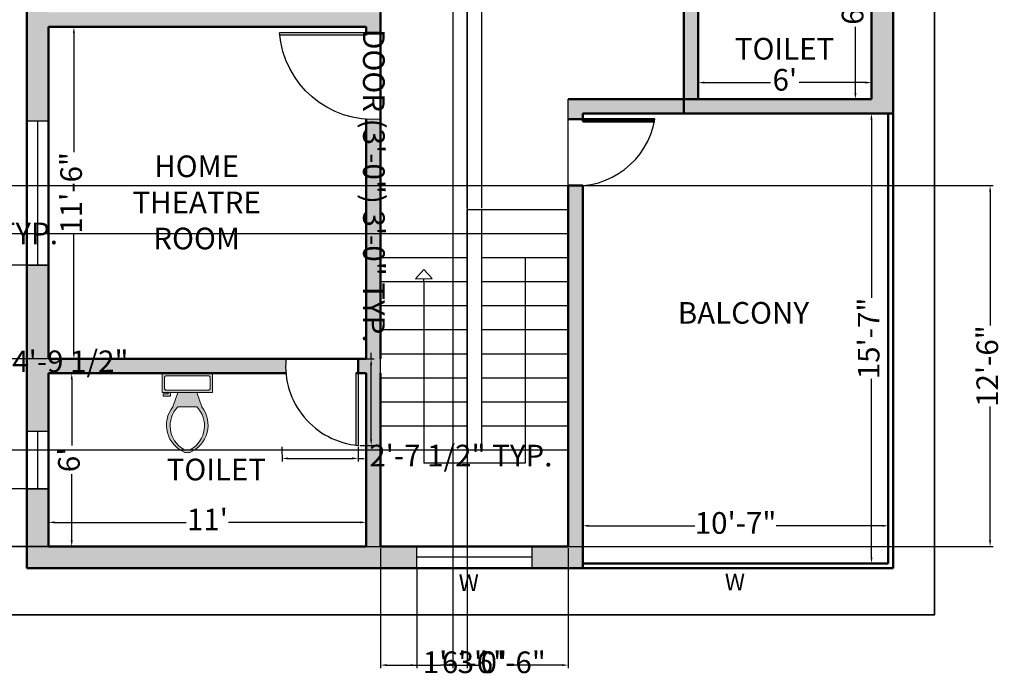
# Model space of a CAD drawing. Units: inches. Extents: x 2463 to 3327, y 6994 to 7582.
# Tile 4 of 5: x 2917 to 3327, y 6995 to 7269. Entities that reach past the tile are written whole.
import ezdxf

# ---------------------------------------------------------------- set-up
doc = ezdxf.new("R2010")
doc.units = ezdxf.units.IN
for name, color, linetype, lineweight in [('A-ANNO-DIMS', 2, 'Continuous', 18), ('A-ANNO-TEXT', 7, 'Continuous', 18), ('A-ANNO-TTLB', 7, 'Continuous', 35), ('A-AREA-IDEN', 3, 'Continuous', 25), ('A-DOOR', 4, 'Continuous', 25), ('A-FLOR-FIXT', 8, 'Continuous', 18), ('A-FLOR-STRS', 3, 'Continuous', 25), ('A-GLAZ', 4, 'Continuous', 25), ('A-WALL', 7, 'Continuous', 50), ('A-WALL-PATT', 252, 'Continuous', 13)]:
    doc.layers.add(name, color=color, linetype=linetype, lineweight=lineweight)
doc.styles.get("Standard").update_dxf_attribs({"font": 'times.ttf'})
doc.dimstyles.new('ISO-25', dxfattribs={"dimtxt": 9, "dimasz": 2.5, "dimexe": 1.25, "dimexo": 0.625, "dimgap": 2, "dimtad": 0, "dimdec": 1, "dimlunit": 4, "dimtxsty": 'Standard', "dimcen": 2.5, "dimadec": 0, "dimazin": 0, "dimtfac": 1, "dimtdec": 1, "dimtmove": 0, "dimatfit": 3, "dimfxl": 1, "dimarcsym": 0})

# ---------------------------------------------------------------- blocks, each defined once
blk = doc.blocks.new('*D17')
at = {"layer": 'A-ANNO-DIMS', "color": 0, "lineweight": -2, "transparency": 16777216}
for p, q in [((3270.8, 7307.83), (3263.49, 7307.83)), ((3264.74, 7305.33), (3264.74, 7277.78)), ((3264.74, 7238.33), (3264.74, 7265.87)), ((3270.8, 7235.83), (3263.49, 7235.83))]:
    blk.add_line(p, q, dxfattribs=at)
at = {"layer": 'A-ANNO-DIMS', "color": 0, "transparency": 16777216}
for points in [[(3264.33, 7305.33), (3265.16, 7305.33), (3264.74, 7307.83)], [(3264.33, 7238.33), (3265.16, 7238.33), (3264.74, 7235.83)]]:
    blk.add_solid(points, dxfattribs=at)
at = {"layer": 'Defpoints', "color": 0, "transparency": 16777216}
for p in [(3264.74, 7307.83), (3271.42, 7307.83), (3271.42, 7235.83)]:
    blk.add_point(p, dxfattribs=at)
at = {"layer": 'A-ANNO-DIMS', "color": 0, "transparency": 16777216, "insert": (3264.74, 7271.83), "char_height": 9, "attachment_point": 5, "rotation": 90}
blk.add_mtext("6'", dxfattribs=at)
blk = doc.blocks.new('*D19')
at = {"layer": 'A-ANNO-DIMS', "color": 0, "lineweight": -2, "transparency": 16777216}
for p, q in [((3199.42, 7236.45), (3199.42, 7243.92)), ((3271.42, 7236.45), (3271.42, 7243.92)), ((3201.92, 7242.67), (3229.47, 7242.67)), ((3268.92, 7242.67), (3241.37, 7242.67))]:
    blk.add_line(p, q, dxfattribs=at)
at = {"layer": 'A-ANNO-DIMS', "color": 0, "transparency": 16777216}
for points in [[(3201.92, 7243.09), (3201.92, 7242.25), (3199.42, 7242.67)], [(3268.92, 7243.09), (3268.92, 7242.25), (3271.42, 7242.67)]]:
    blk.add_solid(points, dxfattribs=at)
at = {"layer": 'Defpoints', "color": 0, "transparency": 16777216}
for p in [(3271.42, 7242.67), (3199.42, 7235.83), (3271.42, 7235.83)]:
    blk.add_point(p, dxfattribs=at)
at = {"layer": 'A-ANNO-DIMS', "color": 0, "transparency": 16777216, "insert": (3235.42, 7242.67), "char_height": 9, "attachment_point": 5}
blk.add_mtext("6'", dxfattribs=at)
blk = doc.blocks.new('*D20')
at = {"layer": 'A-ANNO-DIMS', "color": 0, "lineweight": -2, "transparency": 16777216}
for p, q in [((2929.42, 7050.45), (2929.42, 7061.12)), ((2931.92, 7059.87), (2986.64, 7059.87)), ((3058.92, 7059.87), (3004.2, 7059.87)), ((3061.42, 7050.45), (3061.42, 7061.12))]:
    blk.add_line(p, q, dxfattribs=at)
at = {"layer": 'A-ANNO-DIMS', "color": 0, "transparency": 16777216}
for points in [[(2931.92, 7060.29), (2931.92, 7059.45), (2929.42, 7059.87)], [(3058.92, 7060.29), (3058.92, 7059.45), (3061.42, 7059.87)]]:
    blk.add_solid(points, dxfattribs=at)
at = {"layer": 'Defpoints', "color": 0, "transparency": 16777216}
for p in [(3061.42, 7059.87), (2929.42, 7049.83), (3061.42, 7049.83)]:
    blk.add_point(p, dxfattribs=at)
at = {"layer": 'A-ANNO-DIMS', "color": 0, "transparency": 16777216, "insert": (2995.42, 7059.87), "char_height": 9, "attachment_point": 5}
blk.add_mtext("11'", dxfattribs=at)
blk = doc.blocks.new('*D21')
at = {"layer": 'A-ANNO-DIMS', "color": 0, "lineweight": -2, "transparency": 16777216}
for p, q in [((2930.05, 7121.83), (2940.27, 7121.83)), ((2939.02, 7119.33), (2939.02, 7091.78)), ((2939.02, 7052.33), (2939.02, 7079.87)), ((2930.05, 7049.83), (2940.27, 7049.83))]:
    blk.add_line(p, q, dxfattribs=at)
at = {"layer": 'A-ANNO-DIMS', "color": 0, "transparency": 16777216}
for points in [[(2938.6, 7119.33), (2939.43, 7119.33), (2939.02, 7121.83)], [(2938.6, 7052.33), (2939.43, 7052.33), (2939.02, 7049.83)]]:
    blk.add_solid(points, dxfattribs=at)
at = {"layer": 'Defpoints', "color": 0, "transparency": 16777216}
for p in [(2929.42, 7121.83), (2939.02, 7121.83), (2929.42, 7049.83)]:
    blk.add_point(p, dxfattribs=at)
at = {"layer": 'A-ANNO-DIMS', "color": 0, "transparency": 16777216, "insert": (2939.02, 7085.83), "char_height": 9, "attachment_point": 5, "rotation": 90}
blk.add_mtext("6'", dxfattribs=at)
blk = doc.blocks.new('*D14')
at = {"layer": 'A-ANNO-DIMS', "color": 0, "lineweight": -2, "transparency": 16777216}
for p, q in [((2930.05, 7265.83), (2941.18, 7265.83)), ((2939.93, 7263.33), (2939.93, 7213.69)), ((2939.93, 7130.33), (2939.93, 7179.96)), ((2930.05, 7127.83), (2941.18, 7127.83))]:
    blk.add_line(p, q, dxfattribs=at)
at = {"layer": 'A-ANNO-DIMS', "color": 0, "transparency": 16777216}
for points in [[(2939.51, 7263.33), (2940.34, 7263.33), (2939.93, 7265.83)], [(2939.51, 7130.33), (2940.34, 7130.33), (2939.93, 7127.83)]]:
    blk.add_solid(points, dxfattribs=at)
at = {"layer": 'Defpoints', "color": 0, "transparency": 16777216}
for p in [(2929.42, 7265.83), (2939.93, 7265.83), (2929.42, 7127.83)]:
    blk.add_point(p, dxfattribs=at)
at = {"layer": 'A-ANNO-DIMS', "color": 0, "transparency": 16777216, "insert": (2939.93, 7196.83), "char_height": 9, "attachment_point": 5, "rotation": 90}
blk.add_mtext('11\'-6"', dxfattribs=at)
blk = doc.blocks.new('*U11')
for p, q in [((9.5, -6), (9.5, -2)), ((-8, -8.5), (-8, -8)), ((-7, -8), (-7, -9.5)), ((-4, -8), (-6, -14)), ((4, -8), (6, -14)), ((-10, -8.5), (-8, -8.5)), ((-10, -9.5), (-10, -8.5)), ((-7, -9.5), (-10, -9.5)), ((4, -14), (-4, -14))]:
    blk.add_line(p, q)
blk.add_lwpolyline([(10.5, -8), (10.5, 0), (-10.5, 0), (-10.5, -8)], close=True)
for points in [[(-9.5, -2), (-9.5, -6)], [(8.5, -1), (-8.5, -1)], [(-8.5, -7), (8.5, -7)]]:
    blk.add_lwpolyline(points)
for centre, radius, start, end in [((-8.62, -1.88), 0.884, 81.8699, 188.1301), ((8.62, -1.88), 0.884, 351.8699, 98.1301), ((-8.62, -6.12), 0.884, 171.8699, 278.1301), ((8.62, -6.12), 0.884, 261.8699, 8.1301), ((3.52, -21.58), 12.17, 141.4691, 247.9714), ((4.2, -21.82), 11.33, 136.3677, 238.9468), ((-3.52, -21.58), 12.17, 292.0284, 38.5307), ((-4.2, -21.82), 11.33, 301.053, 43.6321), ((0, -27.88), 4, 245.7318, 294.2682), ((0, -29), 4, 254.8605, 285.1395)]:
    blk.add_arc(centre, radius, start, end)
blk = doc.blocks.new('*D22')
at = {"layer": 'A-ANNO-DIMS', "color": 0, "lineweight": -2, "transparency": 16777216}
for p, q in [((3277.8, 7229.83), (3270.17, 7229.83)), ((3271.42, 7227.33), (3271.42, 7153.19)), ((3271.42, 7045.33), (3271.42, 7119.46)), ((3277.8, 7042.83), (3270.17, 7042.83))]:
    blk.add_line(p, q, dxfattribs=at)
at = {"layer": 'A-ANNO-DIMS', "color": 0, "transparency": 16777216}
for points in [[(3271.01, 7227.33), (3271.84, 7227.33), (3271.42, 7229.83)], [(3271.01, 7045.33), (3271.84, 7045.33), (3271.42, 7042.83)]]:
    blk.add_solid(points, dxfattribs=at)
at = {"layer": 'Defpoints', "color": 0, "transparency": 16777216}
for p in [(3271.42, 7229.83), (3278.42, 7229.83), (3278.42, 7042.83)]:
    blk.add_point(p, dxfattribs=at)
at = {"layer": 'A-ANNO-DIMS', "color": 0, "transparency": 16777216, "insert": (3271.42, 7136.33), "char_height": 9, "attachment_point": 5, "rotation": 90}
blk.add_mtext('15\'-7"', dxfattribs=at)
blk = doc.blocks.new('*D23')
at = {"layer": 'A-ANNO-DIMS', "color": 0, "lineweight": -2, "transparency": 16777216}
for p, q in [((3151.42, 7043.45), (3151.42, 7059.7)), ((3278.42, 7043.45), (3278.42, 7059.7)), ((3153.92, 7058.45), (3198.05, 7058.45)), ((3275.92, 7058.45), (3231.79, 7058.45))]:
    blk.add_line(p, q, dxfattribs=at)
at = {"layer": 'A-ANNO-DIMS', "color": 0, "transparency": 16777216}
for points in [[(3153.92, 7058.87), (3153.92, 7058.03), (3151.42, 7058.45)], [(3275.92, 7058.87), (3275.92, 7058.03), (3278.42, 7058.45)]]:
    blk.add_solid(points, dxfattribs=at)
at = {"layer": 'Defpoints', "color": 0, "transparency": 16777216}
for p in [(3278.42, 7058.45), (3151.42, 7042.83), (3278.42, 7042.83)]:
    blk.add_point(p, dxfattribs=at)
at = {"layer": 'A-ANNO-DIMS', "color": 0, "transparency": 16777216, "insert": (3214.92, 7058.45), "char_height": 9, "attachment_point": 5}
blk.add_mtext('10\'-7"', dxfattribs=at)
blk = doc.blocks.new('DOOR-36')
for p, q in [((0, 6), (0, 42)), ((1, 6), (1, 41.91))]:
    blk.add_line(p, q)
blk.add_arc((-3, 3), 39.12, 355.6013, 85.6013)
blk = doc.blocks.new('DOOR-30')
for p, q in [((29.14, 30), (29.14, 0)), ((30.14, 30), (30.14, 0))]:
    blk.add_line(p, q)
blk.add_arc((33.14, 33), 33.14, 174.8056, 264.8056)
blk = doc.blocks.new('WIN-60')
for p, q in [((9, 60), (0, 60)), ((4.5, 60), (4.5, 0)), ((9, 0), (0, 0))]:
    blk.add_line(p, q)
blk = doc.blocks.new('WIN-24')
for p, q in [((9, 24), (0, 24)), ((4.5, 24), (4.5, 0)), ((9, 0), (0, 0))]:
    blk.add_line(p, q)
blk = doc.blocks.new('WIN-48')
for p, q in [((0, 9), (0, 0)), ((48, 9), (48, 0)), ((0, 4.5), (48, 4.5))]:
    blk.add_line(p, q)
blk = doc.blocks.new('*D35')
at = {"layer": 'A-ANNO-DIMS', "color": 0, "lineweight": -2, "transparency": 16777216}
for p, q in [((2780.62, 7133.65), (2780.62, 7124.39)), ((2838.22, 7133.65), (2838.22, 7124.39)), ((2783.12, 7125.64), (2835.72, 7125.64)), ((2838.22, 7125.64), (2840.72, 7125.64))]:
    blk.add_line(p, q, dxfattribs=at)
at = {"layer": 'A-ANNO-DIMS', "color": 0, "transparency": 16777216}
for points in [[(2783.12, 7126.06), (2783.12, 7125.22), (2780.62, 7125.64)], [(2835.72, 7126.06), (2835.72, 7125.22), (2838.22, 7125.64)]]:
    blk.add_solid(points, dxfattribs=at)
at = {"layer": 'Defpoints', "color": 0, "transparency": 16777216}
for p in [(2780.62, 7134.28), (2838.22, 7134.28), (2838.22, 7125.64)]:
    blk.add_point(p, dxfattribs=at)
at = {"layer": 'A-ANNO-DIMS', "color": 0, "transparency": 16777216, "insert": (2903.83, 7125.64), "char_height": 9, "attachment_point": 5}
blk.add_mtext('DINING SET 4\'-9 1/2"', dxfattribs=at)
blk = doc.blocks.new('*D38')
at = {"layer": 'A-ANNO-DIMS', "color": 0, "lineweight": -2, "transparency": 16777216}
for p, q in [((2864.43, 7170.45), (2864.43, 7180.08)), ((2866.93, 7178.83), (2870.93, 7178.83)), ((2873.43, 7170.45), (2873.43, 7180.08)), ((2873.43, 7178.83), (2875.93, 7178.83))]:
    blk.add_line(p, q, dxfattribs=at)
at = {"layer": 'A-ANNO-DIMS', "color": 0, "transparency": 16777216}
for points in [[(2866.93, 7179.24), (2866.93, 7178.41), (2864.43, 7178.83)], [(2870.93, 7179.24), (2870.93, 7178.41), (2873.43, 7178.83)]]:
    blk.add_solid(points, dxfattribs=at)
at = {"layer": 'Defpoints', "color": 0, "transparency": 16777216}
for p in [(2873.43, 7178.83), (2864.43, 7169.83), (2873.43, 7169.83)]:
    blk.add_point(p, dxfattribs=at)
at = {"layer": 'A-ANNO-DIMS', "color": 0, "transparency": 16777216, "insert": (2905.86, 7178.83), "char_height": 9, "attachment_point": 5}
blk.add_mtext('0\'-9" TYP.', dxfattribs=at)
blk = doc.blocks.new('*D43')
at = {"layer": 'A-ANNO-DIMS', "color": 0, "lineweight": -2, "transparency": 16777216}
for p, q in [((3063.47, 7127.84), (3063.47, 7130.34)), ((3058.69, 7127.84), (3064.72, 7127.85)), ((3063.48, 7094.34), (3063.47, 7125.34)), ((3058.71, 7091.84), (3064.73, 7091.85))]:
    blk.add_line(p, q, dxfattribs=at)
at = {"layer": 'A-ANNO-DIMS', "color": 0, "transparency": 16777216}
for points in [[(3063.88, 7125.34), (3063.05, 7125.34), (3063.47, 7127.84)], [(3063.9, 7094.34), (3063.06, 7094.34), (3063.48, 7091.84)]]:
    blk.add_solid(points, dxfattribs=at)
at = {"layer": 'Defpoints', "color": 0, "transparency": 16777216}
for p in [(3058.07, 7127.84), (3063.47, 7127.84), (3058.08, 7091.84)]:
    blk.add_point(p, dxfattribs=at)
at = {"layer": 'A-ANNO-DIMS', "color": 0, "transparency": 16777216, "insert": (3063.44, 7199.74), "char_height": 9, "attachment_point": 5, "rotation": 270.023}
blk.add_mtext('DOOR (3\'-0") 3\'-0" TYP.', dxfattribs=at)
blk = doc.blocks.new('*D44')
at = {"layer": 'A-ANNO-DIMS', "color": 0, "lineweight": -2, "transparency": 16777216}
for p, q in [((3026.42, 7091.2), (3026.43, 7085.18)), ((3058.08, 7091.22), (3058.08, 7085.19)), ((3028.93, 7086.43), (3055.58, 7086.44)), ((3058.08, 7086.44), (3060.58, 7086.44))]:
    blk.add_line(p, q, dxfattribs=at)
at = {"layer": 'A-ANNO-DIMS', "color": 0, "transparency": 16777216}
for points in [[(3028.93, 7086.85), (3028.93, 7086.01), (3026.43, 7086.43)], [(3055.58, 7086.86), (3055.58, 7086.02), (3058.08, 7086.44)]]:
    blk.add_solid(points, dxfattribs=at)
at = {"layer": 'Defpoints', "color": 0, "transparency": 16777216}
for p in [(3026.42, 7091.83), (3058.08, 7091.84), (3058.08, 7086.44)]:
    blk.add_point(p, dxfattribs=at)
at = {"layer": 'A-ANNO-DIMS', "color": 0, "transparency": 16777216, "insert": (3100.76, 7086.46), "char_height": 9, "attachment_point": 5, "rotation": 0.023}
blk.add_mtext('2\'-7 1/2" TYP.', dxfattribs=at)
blk = doc.blocks.new('*D59')
at = {"layer": 'A-ANNO-DIMS', "color": 0, "lineweight": -2, "transparency": 16777216}
for p, q in [((2745.06, 7199.83), (3321.97, 7199.83)), ((3320.72, 7197.33), (3320.72, 7141.69)), ((3320.72, 7052.33), (3320.72, 7107.96)), ((2745.06, 7049.83), (3321.97, 7049.83))]:
    blk.add_line(p, q, dxfattribs=at)
at = {"layer": 'A-ANNO-DIMS', "color": 0, "transparency": 16777216}
for points in [[(3320.31, 7197.33), (3321.14, 7197.33), (3320.72, 7199.83)], [(3320.31, 7052.33), (3321.14, 7052.33), (3320.72, 7049.83)]]:
    blk.add_solid(points, dxfattribs=at)
at = {"layer": 'Defpoints', "color": 0, "transparency": 16777216}
for p in [(2744.43, 7199.83), (2744.43, 7049.83), (3320.72, 7049.83)]:
    blk.add_point(p, dxfattribs=at)
at = {"layer": 'A-ANNO-DIMS', "color": 0, "transparency": 16777216, "insert": (3320.72, 7124.83), "char_height": 9, "attachment_point": 5, "rotation": 90}
blk.add_mtext('12\'-6"', dxfattribs=at)
blk = doc.blocks.new('*D68')
at = {"layer": 'A-ANNO-DIMS', "color": 0, "lineweight": -2, "transparency": 16777216}
for p, q in [((3103.42, 7391.2), (3103.42, 6999.28)), ((3097.42, 7385.2), (3097.42, 6999.28)), ((3094.92, 7000.53), (3092.42, 7000.53)), ((3097.42, 7000.53), (3103.42, 7000.53)), ((3105.92, 7000.53), (3108.42, 7000.53))]:
    blk.add_line(p, q, dxfattribs=at)
at = {"layer": 'A-ANNO-DIMS', "color": 0, "transparency": 16777216}
for points in [[(3094.92, 7000.94), (3094.92, 7000.11), (3097.42, 7000.53)], [(3105.92, 7000.94), (3105.92, 7000.11), (3103.42, 7000.53)]]:
    blk.add_solid(points, dxfattribs=at)
at = {"layer": 'Defpoints', "color": 0, "transparency": 16777216}
for p in [(3103.42, 7391.83), (3097.42, 7385.83), (3103.42, 7000.53)]:
    blk.add_point(p, dxfattribs=at)
at = {"layer": 'A-ANNO-DIMS', "color": 0, "transparency": 16777216, "insert": (3122.51, 7000.53), "char_height": 9, "attachment_point": 5}
blk.add_mtext('0\'-6"', dxfattribs=at)
blk = doc.blocks.new('*D71')
at = {"layer": 'A-ANNO-DIMS', "color": 0, "lineweight": -2, "transparency": 16777216}
for p, q in [((3067.42, 7272.45), (3067.42, 7562.38)), ((3069.92, 7561.13), (3113.55, 7561.13)), ((3190.92, 7561.13), (3147.29, 7561.13)), ((3193.42, 7230.45), (3193.42, 7562.38))]:
    blk.add_line(p, q, dxfattribs=at)
at = {"layer": 'A-ANNO-DIMS', "color": 0, "transparency": 16777216}
for points in [[(3069.92, 7561.54), (3069.92, 7560.71), (3067.42, 7561.13)], [(3190.92, 7561.54), (3190.92, 7560.71), (3193.42, 7561.13)]]:
    blk.add_solid(points, dxfattribs=at)
at = {"layer": 'Defpoints', "color": 0, "transparency": 16777216}
for p in [(3193.42, 7561.13), (3067.42, 7271.83), (3193.42, 7229.83)]:
    blk.add_point(p, dxfattribs=at)
at = {"layer": 'A-ANNO-DIMS', "color": 0, "transparency": 16777216, "insert": (3130.42, 7561.13), "char_height": 9, "attachment_point": 5}
blk.add_mtext('10\'-6"', dxfattribs=at)
blk = doc.blocks.new('*D72')
at = {"layer": 'A-ANNO-DIMS', "color": 0, "lineweight": -2, "transparency": 16777216}
for p, q in [((3067.42, 7049.2), (3067.42, 6999.28)), ((3145.42, 7049.2), (3145.42, 6999.28)), ((3069.92, 7000.53), (3092.38, 7000.53)), ((3142.92, 7000.53), (3120.46, 7000.53))]:
    blk.add_line(p, q, dxfattribs=at)
at = {"layer": 'A-ANNO-DIMS', "color": 0, "transparency": 16777216}
for points in [[(3069.92, 7000.94), (3069.92, 7000.11), (3067.42, 7000.53)], [(3142.92, 7000.94), (3142.92, 7000.11), (3145.42, 7000.53)]]:
    blk.add_solid(points, dxfattribs=at)
at = {"layer": 'Defpoints', "color": 0, "transparency": 16777216}
for p in [(3067.42, 7049.83), (3145.42, 7049.83), (3145.42, 7000.53)]:
    blk.add_point(p, dxfattribs=at)
at = {"layer": 'A-ANNO-DIMS', "color": 0, "transparency": 16777216, "insert": (3106.42, 7000.53), "char_height": 9, "attachment_point": 5}
blk.add_mtext('6\'-6"', dxfattribs=at)
blk = doc.blocks.new('*D73')
at = {"layer": 'A-ANNO-DIMS', "color": 0, "lineweight": -2, "transparency": 16777216}
for p, q in [((3064.92, 7561.13), (3062.42, 7561.13)), ((3067.42, 7180.45), (3067.42, 7562.38)), ((3067.42, 7561.13), (3071.37, 7561.13)), ((3103.42, 7561.13), (3099.48, 7561.13)), ((3103.42, 7190.45), (3103.42, 7562.38)), ((3105.92, 7561.13), (3108.42, 7561.13))]:
    blk.add_line(p, q, dxfattribs=at)
at = {"layer": 'A-ANNO-DIMS', "color": 0, "transparency": 16777216}
for points in [[(3064.92, 7561.54), (3064.92, 7560.71), (3067.42, 7561.13)], [(3105.92, 7561.54), (3105.92, 7560.71), (3103.42, 7561.13)]]:
    blk.add_solid(points, dxfattribs=at)
at = {"layer": 'Defpoints', "color": 0, "transparency": 16777216}
for p in [(3103.42, 7561.13), (3103.42, 7189.83), (3067.42, 7179.83)]:
    blk.add_point(p, dxfattribs=at)
at = {"layer": 'A-ANNO-DIMS', "color": 0, "transparency": 16777216, "insert": (3085.42, 7561.13), "char_height": 9, "attachment_point": 5}
blk.add_mtext('3\'-0"', dxfattribs=at)
blk = doc.blocks.new('*D74')
at = {"layer": 'A-ANNO-DIMS', "color": 0, "lineweight": -2, "transparency": 16777216}
for p, q in [((3100.92, 7561.13), (3098.42, 7561.13)), ((3103.42, 7190.45), (3103.42, 7562.38)), ((3103.42, 7561.13), (3109.42, 7561.13)), ((3109.42, 7190.45), (3109.42, 7562.38)), ((3111.92, 7561.13), (3114.42, 7561.13))]:
    blk.add_line(p, q, dxfattribs=at)
at = {"layer": 'A-ANNO-DIMS', "color": 0, "transparency": 16777216}
for points in [[(3100.92, 7561.54), (3100.92, 7560.71), (3103.42, 7561.13)], [(3111.92, 7561.54), (3111.92, 7560.71), (3109.42, 7561.13)]]:
    blk.add_solid(points, dxfattribs=at)
at = {"layer": 'Defpoints', "color": 0, "transparency": 16777216}
for p in [(3109.42, 7561.13), (3103.42, 7189.83), (3109.42, 7189.83)]:
    blk.add_point(p, dxfattribs=at)
at = {"layer": 'A-ANNO-DIMS', "color": 0, "transparency": 16777216, "insert": (3128.51, 7561.13), "char_height": 9, "attachment_point": 5}
blk.add_mtext('0\'-6"', dxfattribs=at)
blk = doc.blocks.new('*D75')
at = {"layer": 'A-ANNO-DIMS', "color": 0, "lineweight": -2, "transparency": 16777216}
for p, q in [((3144.8, 7179.83), (2471.88, 7179.83)), ((2473.13, 7177.33), (2473.13, 7148.9)), ((2473.13, 7092.33), (2473.13, 7120.75)), ((3144.8, 7089.83), (2471.88, 7089.83))]:
    blk.add_line(p, q, dxfattribs=at)
at = {"layer": 'A-ANNO-DIMS', "color": 0, "transparency": 16777216}
for points in [[(2472.71, 7177.33), (2473.55, 7177.33), (2473.13, 7179.83)], [(2472.71, 7092.33), (2473.55, 7092.33), (2473.13, 7089.83)]]:
    blk.add_solid(points, dxfattribs=at)
at = {"layer": 'Defpoints', "color": 0, "transparency": 16777216}
for p in [(3145.42, 7179.83), (2473.13, 7089.83), (3145.42, 7089.83)]:
    blk.add_point(p, dxfattribs=at)
at = {"layer": 'A-ANNO-DIMS', "color": 0, "transparency": 16777216, "insert": (2473.13, 7134.83), "char_height": 9, "attachment_point": 5, "rotation": 90}
blk.add_mtext('7\'-6"', dxfattribs=at)
blk = doc.blocks.new('*D76')
at = {"layer": 'A-ANNO-DIMS', "color": 0, "lineweight": -2, "transparency": 16777216}
for p, q in [((2473.13, 7073.83), (2473.13, 7076.33)), ((2928.8, 7073.83), (2471.88, 7073.83)), ((2473.13, 7052.33), (2473.13, 7071.33)), ((2928.8, 7049.83), (2471.88, 7049.83))]:
    blk.add_line(p, q, dxfattribs=at)
at = {"layer": 'A-ANNO-DIMS', "color": 0, "transparency": 16777216}
for points in [[(2472.71, 7071.33), (2473.55, 7071.33), (2473.13, 7073.83)], [(2472.71, 7052.33), (2473.55, 7052.33), (2473.13, 7049.83)]]:
    blk.add_solid(points, dxfattribs=at)
at = {"layer": 'Defpoints', "color": 0, "transparency": 16777216}
for p in [(2473.13, 7073.83), (2929.42, 7073.83), (2929.42, 7049.83)]:
    blk.add_point(p, dxfattribs=at)
at = {"layer": 'A-ANNO-DIMS', "color": 0, "transparency": 16777216, "insert": (2473.13, 7090.51), "char_height": 9, "attachment_point": 5, "rotation": 90}
blk.add_mtext('2\'-0"', dxfattribs=at)
blk = doc.blocks.new('*D77')
at = {"layer": 'A-ANNO-DIMS', "color": 0, "lineweight": -2, "transparency": 16777216}
for p, q in [((2928.8, 7166.83), (2471.88, 7166.83)), ((2473.13, 7164.33), (2473.13, 7161.38)), ((2473.13, 7130.33), (2473.13, 7133.27)), ((2928.8, 7127.83), (2471.88, 7127.83))]:
    blk.add_line(p, q, dxfattribs=at)
at = {"layer": 'A-ANNO-DIMS', "color": 0, "transparency": 16777216}
for points in [[(2472.71, 7164.33), (2473.55, 7164.33), (2473.13, 7166.83)], [(2472.71, 7130.33), (2473.55, 7130.33), (2473.13, 7127.83)]]:
    blk.add_solid(points, dxfattribs=at)
at = {"layer": 'Defpoints', "color": 0, "transparency": 16777216}
for p in [(2473.13, 7166.83), (2929.42, 7166.83), (2929.42, 7127.83)]:
    blk.add_point(p, dxfattribs=at)
at = {"layer": 'A-ANNO-DIMS', "color": 0, "transparency": 16777216, "insert": (2473.13, 7147.33), "char_height": 9, "attachment_point": 5, "rotation": 90}
blk.add_mtext('3\'-3"', dxfattribs=at)
blk = doc.blocks.new('*D81')
at = {"layer": 'A-ANNO-DIMS', "color": 0, "lineweight": -2, "transparency": 16777216}
for p, q in [((3067.42, 7049.2), (3067.42, 6999.28)), ((3082.42, 7040.2), (3082.42, 6999.28)), ((3069.92, 7000.53), (3079.92, 7000.53)), ((3082.42, 7000.53), (3084.92, 7000.53))]:
    blk.add_line(p, q, dxfattribs=at)
at = {"layer": 'A-ANNO-DIMS', "color": 0, "transparency": 16777216}
for points in [[(3069.92, 7000.94), (3069.92, 7000.11), (3067.42, 7000.53)], [(3079.92, 7000.94), (3079.92, 7000.11), (3082.42, 7000.53)]]:
    blk.add_solid(points, dxfattribs=at)
at = {"layer": 'Defpoints', "color": 0, "transparency": 16777216}
for p in [(3067.42, 7049.83), (3082.42, 7040.83), (3082.42, 7000.53)]:
    blk.add_point(p, dxfattribs=at)
at = {"layer": 'A-ANNO-DIMS', "color": 0, "transparency": 16777216, "insert": (3098.47, 7000.53), "char_height": 9, "attachment_point": 5}
blk.add_mtext('1\'-3"', dxfattribs=at)

msp = doc.modelspace()

# ---------------------------------------------------------------- hatches: boundary and pattern name
at = {"layer": 'A-WALL-PATT'}
h = msp.add_hatch(color=256, dxfattribs=at)
h.dxf.hatch_style = 1
h.paths.add_polyline_path([(2522.43, 7511.83), (2690.43, 7511.83), (2690.43, 7385.83), (2696.43, 7385.83), (2702.68, 7385.83), (2702.68, 7391.83), (2696.43, 7391.83), (2696.43, 7511.83), (2864.43, 7511.83), (2864.43, 7481.83), (2873.43, 7481.83), (2873.43, 7520.83), (2513.43, 7520.83), (2513.43, 7501.71), (2522.43, 7501.71)])
h.paths.add_polyline_path([(2522.43, 7453.71, -0.042779), (2513.43, 7453.71), (2513.43, 7392.77), (2522.43, 7392.77)], flags=0)
h.paths.add_polyline_path([(2522.43, 7332.77), (2513.43, 7332.77), (2513.43, 7226.83), (2522.43, 7226.83), (2522.43, 7265.83), (2654.43, 7265.83), (2654.43, 7263.42), (2660.43, 7263.42), (2660.43, 7271.83), (2522.43, 7271.83)])
h.paths.add_polyline_path([(2873.43, 7421.83), (2864.43, 7421.83), (2864.43, 7391.83), (2861.59, 7391.83), (2861.59, 7385.83), (2864.43, 7385.83), (2864.43, 7361.83), (2873.43, 7361.83)])
h.paths.add_polyline_path([(2792.43, 7385.83), (2831.59, 7385.83, -0.045361), (2831.59, 7391.83), (2738.68, 7391.83, -0.038405), (2738.68, 7385.83), (2786.43, 7385.83), (2786.43, 7313.83), (2786.43, 7307.83), (2786.43, 7305.07), (2792.43, 7305.07), (2792.43, 7307.83), (2864.43, 7307.83), (2864.43, 7235.83), (2792.43, 7235.83), (2792.43, 7275.07, -0.045361), (2786.43, 7275.07), (2786.43, 7235.83), (2786.43, 7229.83), (2864.43, 7229.83), (2864.43, 7169.83), (2873.43, 7169.83), (2873.43, 7337.83), (2864.43, 7337.83), (2864.43, 7313.83), (2792.43, 7313.83)])
h.paths.add_polyline_path([(2873.43, 7109.83), (2864.43, 7109.83), (2864.43, 7049.83), (2834.43, 7049.83), (2834.43, 7040.83), (2873.43, 7040.83)])
h.paths.add_polyline_path([(2774.43, 7049.83), (2744.43, 7049.83), (2744.43, 7199.83), (2738.43, 7199.83), (2738.43, 7049.83), (2723.43, 7049.83), (2723.43, 7040.83), (2774.43, 7040.83)])
h.paths.add_polyline_path([(2675.43, 7049.83), (2660.43, 7049.83), (2660.43, 7121.83), (2660.43, 7127.83), (2660.43, 7227.42, -0.038405), (2654.43, 7227.42), (2654.43, 7127.83), (2651.08, 7127.83), (2651.08, 7121.83), (2654.43, 7121.83), (2654.43, 7049.83), (2522.43, 7049.83), (2522.43, 7073.83), (2513.43, 7073.83), (2513.43, 7040.83), (2675.43, 7040.83)])
h.paths.add_polyline_path([(2621.08, 7127.83), (2522.43, 7127.83), (2522.43, 7166.83), (2513.43, 7166.83), (2513.43, 7097.83), (2522.43, 7097.83), (2522.43, 7121.83), (2621.08, 7121.83, -0.045361)], flags=17)
h.paths.add_polyline_path([(3280.42, 7520.83), (2920.42, 7520.83), (2920.42, 7501.71), (2929.42, 7501.71), (2929.42, 7511.83), (3097.42, 7511.83), (3097.42, 7385.83), (3103.42, 7385.83), (3109.67, 7385.83), (3109.67, 7391.83), (3103.42, 7391.83), (3103.42, 7511.83), (3271.42, 7511.83), (3271.42, 7481.83), (3280.42, 7481.83)])
h.paths.add_polyline_path([(3280.42, 7421.83), (3271.42, 7421.83), (3271.42, 7391.83), (3268.58, 7391.83), (3268.58, 7385.83), (3271.42, 7385.83), (3271.42, 7361.83), (3280.42, 7361.83)])
h.paths.add_polyline_path([(3238.58, 7391.83), (3145.67, 7391.83, -0.038405), (3145.67, 7385.83), (3193.42, 7385.83), (3193.42, 7313.83), (3193.42, 7307.83), (3193.42, 7305.07), (3199.42, 7305.07), (3199.42, 7307.83), (3271.42, 7307.83), (3271.42, 7235.83), (3199.42, 7235.83), (3193.42, 7235.83), (3193.42, 7229.83), (3271.42, 7229.83), (3280.42, 7229.83), (3280.42, 7337.83), (3271.42, 7337.83), (3271.42, 7313.83), (3199.42, 7313.83), (3199.42, 7385.83), (3238.58, 7385.83, -0.045361)])
h.paths.add_polyline_path([(3199.42, 7275.07, -0.045361), (3193.42, 7275.07), (3193.42, 7235.83), (3199.42, 7235.83)], flags=17)
h.paths.add_polyline_path([(3193.42, 7235.83), (3145.42, 7235.83), (3145.42, 7227.44), (3151.42, 7227.44), (3151.42, 7229.83), (3193.42, 7229.83)])
h.paths.add_polyline_path([(3151.42, 7199.83, -0.044871), (3145.42, 7199.83), (3145.42, 7049.83), (3130.42, 7049.83), (3130.42, 7040.83), (3151.42, 7040.83), (3151.42, 7049.83)])
h.paths.add_polyline_path([(3082.42, 7049.83), (3067.42, 7049.83), (3067.42, 7121.83), (3067.42, 7127.83), (3067.42, 7227.42, -0.038405), (3061.42, 7227.42), (3061.42, 7127.83), (3058.07, 7127.83), (3058.07, 7121.83), (3061.42, 7121.83), (3061.42, 7049.83), (2929.42, 7049.83), (2929.42, 7073.83), (2920.42, 7073.83), (2920.42, 7040.83), (3082.42, 7040.83)])
h.paths.add_polyline_path([(3028.07, 7121.83), (2997.56, 7121.83), (2997.56, 7113.83), (2991.06, 7113.83), (2993.06, 7107.83, -0.501323), (2988.1, 7088.96, -0.132891), (2986.01, 7088.96, -0.501317), (2981.06, 7107.83), (2983.06, 7113.83), (2980.06, 7113.83), (2980.06, 7112.33), (2977.06, 7112.33), (2977.06, 7113.83), (2976.56, 7113.83), (2976.56, 7121.83), (2929.42, 7121.83), (2929.42, 7097.83), (2920.42, 7097.83), (2920.42, 7166.83), (2929.42, 7166.83), (2929.42, 7127.83), (3028.07, 7127.83, 0.045361)], flags=17)
h.paths.add_polyline_path([(2995.56, 7120.83, -0.414214), (2996.56, 7120.08), (2996.56, 7115.83, -0.414214), (2995.81, 7114.83), (2978.56, 7114.83, -0.414214), (2977.56, 7115.58), (2977.56, 7119.83, -0.414214), (2978.31, 7120.83)], flags=16)
h.paths.add_polyline_path([(2988.7, 7090.3, -0.215004), (2985.41, 7090.3, -0.48008), (2983.06, 7107.83), (2991.06, 7107.83, -0.48008)], flags=16)
h.paths.add_polyline_path([(2929.42, 7265.83), (3061.42, 7265.83), (3061.42, 7263.42), (3067.42, 7263.42), (3067.42, 7271.83), (2929.42, 7271.83), (2929.42, 7332.77), (2920.42, 7332.77), (2920.42, 7226.83), (2929.42, 7226.83)])
h.paths.add_polyline_path([(2929.42, 7453.71, -0.042779), (2920.42, 7453.71), (2920.42, 7392.77), (2929.42, 7392.77)], flags=0)

# ---------------------------------------------------------------- linework, layer by layer
at = {"layer": 'A-ANNO-TTLB'}
msp.add_lwpolyline([(2463.47, 7549.29), (3297.67, 7549.29), (3297.67, 7021.48), (2463.47, 7021.48)], close=True, dxfattribs=at)
at = {"layer": 'A-DOOR'}
msp.add_line((3145.42, 7199.83), (3145.42, 7235.83), dxfattribs=at)
msp.add_arc((3148.42, 7233.19), 33.5, 264.8616, 350.122, dxfattribs=at)
at = {"layer": 'A-FLOR-STRS'}
for p, q in [((3103.42, 7089.83), (3103.42, 7189.83)), ((3109.42, 7189.83), (3103.42, 7189.83)), ((3109.42, 7089.83), (3109.42, 7189.83)), ((3145.42, 7189.83), (3109.42, 7189.83)), ((3103.42, 7179.83), (3067.42, 7179.83)), ((3145.42, 7179.83), (3109.42, 7179.83)), ((3103.42, 7169.83), (3067.42, 7169.83)), ((3145.42, 7169.83), (3109.42, 7169.83)), ((3127.42, 7169.83), (3127.42, 7084.53)), ((3085.42, 7164.96), (3081.96, 7161.1)), ((3088.87, 7161.23), (3085.42, 7164.96)), ((3103.42, 7159.83), (3067.42, 7159.83)), ((3081.96, 7161.1), (3088.87, 7161.23)), ((3085.42, 7159.83), (3085.42, 7161.17)), ((3085.42, 7159.83), (3085.42, 7084.53)), ((3145.42, 7159.83), (3109.42, 7159.83)), ((3103.42, 7149.83), (3067.42, 7149.83)), ((3145.42, 7149.83), (3109.42, 7149.83)), ((3103.42, 7139.83), (3067.42, 7139.83)), ((3145.42, 7139.83), (3109.42, 7139.83)), ((3103.42, 7129.83), (3067.42, 7129.83)), ((3145.42, 7129.83), (3109.42, 7129.83)), ((3067.42, 7121.83), (3067.42, 7127.83)), ((3103.42, 7119.83), (3067.42, 7119.83)), ((3145.42, 7119.83), (3109.42, 7119.83)), ((3103.42, 7109.83), (3067.42, 7109.83)), ((3145.42, 7109.83), (3109.42, 7109.83)), ((3103.42, 7099.83), (3067.42, 7099.83)), ((3145.42, 7099.83), (3109.42, 7099.83)), ((3145.42, 7089.83), (3067.42, 7089.83)), ((3127.42, 7084.53), (3085.42, 7084.53))]:
    msp.add_line(p, q, dxfattribs=at)
at = {"layer": 'A-WALL'}
for p, q in [((2920.42, 7040.83), (2920.42, 7520.83)), ((3280.42, 7520.83), (3280.42, 7040.83)), ((3193.42, 7307.83), (3193.42, 7235.83)), ((3271.42, 7307.83), (3271.42, 7235.83)), ((3199.42, 7275.07), (3199.42, 7235.83)), ((3067.42, 7127.83), (3067.42, 7271.83)), ((3061.42, 7265.83), (2929.42, 7265.83)), ((2929.42, 7127.83), (2929.42, 7265.83)), ((3061.42, 7262.42), (3061.42, 7265.83)), ((3061.42, 7263.42), (3067.42, 7263.42)), ((3199.42, 7235.83), (3145.42, 7235.83)), ((3193.42, 7235.83), (3193.42, 7229.83)), ((3199.42, 7235.83), (3271.42, 7235.83)), ((3061.42, 7127.83), (3061.42, 7227.42)), ((3151.42, 7227.44), (3145.42, 7227.44)), ((3151.42, 7226.44), (3151.42, 7229.83)), ((3193.42, 7229.83), (3151.42, 7229.83)), ((3151.42, 7227.44), (3181.42, 7227.44)), ((3193.42, 7229.83), (3271.42, 7229.83)), ((3271.42, 7229.83), (3280.42, 7229.83)), ((3278.42, 7229.83), (3278.42, 7042.83)), ((3151.42, 7226.44), (3181.42, 7226.44)), ((3145.42, 7199.83), (3145.42, 7049.83)), ((3145.42, 7199.83), (3151.42, 7199.83)), ((3151.42, 7199.83), (3151.42, 7049.83)), ((3061.42, 7127.83), (2929.42, 7127.83)), ((3058.07, 7127.83), (3058.07, 7121.83)), ((3028.07, 7121.83), (2929.42, 7121.83)), ((2929.42, 7049.83), (2929.42, 7121.83)), ((3061.42, 7121.83), (3057.07, 7121.83)), ((3061.42, 7049.83), (3061.42, 7121.83)), ((3067.42, 7049.83), (3067.42, 7121.83)), ((3061.42, 7049.83), (2929.42, 7049.83)), ((3145.42, 7049.83), (3067.42, 7049.83)), ((3151.42, 7049.83), (3151.42, 7040.83)), ((3278.42, 7042.83), (3151.42, 7042.83)), ((3280.42, 7040.83), (2920.42, 7040.83))]:
    msp.add_line(p, q, dxfattribs=at)

# ---------------------------------------------------------------- block references
at = {"layer": 'A-DOOR', "extrusion": (0, 0, -1), "zscale": -1, "rotation": 270.0000000000147}
msp.add_blockref('DOOR-36', (-3067.42, 7263.42), dxfattribs=at)
at = {"layer": 'A-DOOR', "rotation": 0.0230106322837906}
msp.add_blockref('DOOR-30', (3027.95, 7091.83), dxfattribs=at)
at = {"layer": 'A-FLOR-FIXT'}
msp.add_blockref('*U11', (2987.06, 7121.83), dxfattribs=at)
at = {"layer": 'A-GLAZ', "rotation": 180}
for name, p in [('WIN-60', (2929.42, 7226.83)), ('WIN-24', (2929.42, 7097.83)), ('WIN-48', (3130.42, 7049.83))]:
    msp.add_blockref(name, p, dxfattribs=at)

# ---------------------------------------------------------------- texts
at = {"layer": 'A-ANNO-TEXT', "char_height": 7, "attachment_point": 1}
for insert in [(3089.85, 7038.27), (3200.47, 7038.56)]:
    msp.add_mtext_dynamic_manual_height_columns('\\pxqc;{\\fTimes New Roman|b1|i0|c0|p18;W}', width=28.3852, gutter_width=12.5, heights=[0], dxfattribs=dict(at, insert=insert))
at = {"layer": 'A-AREA-IDEN', "char_height": 9, "attachment_point": 1}
for s, width, insert in [('\\pxqc;{\\fTimes New Roman|b1|i0|c0|p18;TOILET}', 62.7452, (3203.92, 7261.23)), ('\\pxqc;{\\fTimes New Roman|b1|i0|c0|p18;HOME \\PTHEATRE\\PROOM}', 97.7954, (2942.03, 7212.37)), ('\\pxqc;{\\fTimes New Roman|b1|i0|c0|p18;BALCONY}', 79.7182, (3178.34, 7151.45)), ('\\pxqc;{\\fTimes New Roman|b1|i0|c0|p18;TOILET}', 69.3628, (2964.46, 7086.34))]:
    msp.add_mtext_dynamic_manual_height_columns(s, width=width, gutter_width=12.5, heights=[0], dxfattribs=dict(at, insert=insert))

# ---------------------------------------------------------------- dimensions: what is measured, and where the dimension line sits
at = {"layer": 'A-ANNO-DIMS'}
for base, p1, p2, override, picture, middle in [((3103.42, 7561.13), (3067.42, 7179.83), (3103.42, 7189.83), {"dimdec": 1, "dimlfac": 1, "dimrnd": 0, "dimzin": 1, "dimdsep": 46, "dimlunit": 4, "dimfrac": 2}, '*D73', (3085.42, 7561.13)), ((3193.42, 7561.13), (3067.42, 7271.83), (3193.42, 7229.83), {"dimdec": 1, "dimlfac": 1, "dimrnd": 0, "dimzin": 1, "dimdsep": 46, "dimlunit": 4, "dimfrac": 2}, '*D71', (3130.42, 7561.13)), ((3109.42, 7561.13), (3103.42, 7189.83), (3109.42, 7189.83), {"dimdec": 1, "dimlfac": 1, "dimrnd": 0, "dimzin": 1, "dimdsep": 46, "dimlunit": 4, "dimfrac": 2}, '*D74', (3128.51, 7561.13)), ((3103.42, 7000.53), (3097.42, 7385.83), (3103.42, 7391.83), {"dimdec": 1, "dimlfac": 1, "dimrnd": 0, "dimzin": 1, "dimdsep": 46, "dimlunit": 4, "dimfrac": 2}, '*D68', (3122.51, 7000.53)), ((3271.42, 7242.67), (3199.42, 7235.83), (3271.42, 7235.83), {"dimclrd": 0, "dimclre": 0, "dimclrt": 0}, '*D19', (3235.42, 7242.67)), ((3061.42, 7059.87), (2929.42, 7049.83), (3061.42, 7049.83), {"dimclrd": 0, "dimclre": 0, "dimclrt": 0}, '*D20', (2995.42, 7059.87)), ((3278.42, 7058.45), (3151.42, 7042.83), (3278.42, 7042.83), {"dimclrd": 0, "dimclre": 0, "dimclrt": 0}, '*D23', (3214.92, 7058.45)), ((3145.42, 7000.53), (3067.42, 7049.83), (3145.42, 7049.83), {"dimdec": 1, "dimlfac": 1, "dimrnd": 0, "dimzin": 1, "dimdsep": 46, "dimlunit": 4, "dimfrac": 2}, '*D72', (3106.42, 7000.53)), ((3082.42, 7000.53), (3067.42, 7049.83), (3082.42, 7040.83), {"dimdec": 1, "dimlfac": 1, "dimrnd": 0, "dimzin": 1, "dimdsep": 46, "dimlunit": 4, "dimfrac": 2}, '*D81', (3098.47, 7000.53))]:
    dim = msp.add_linear_dim(base=base, p1=p1, p2=p2, dimstyle='ISO-25', override=override, dxfattribs=at)
    dim.commit()
    dim.dimension.update_dxf_attribs({"geometry": picture, "text_midpoint": middle})
for base, p1, p2, override, picture, middle in [((3264.74, 7307.83), (3271.42, 7235.83), (3271.42, 7307.83), {"dimclrd": 0, "dimclre": 0, "dimclrt": 0}, '*D17', (3264.74, 7271.83)), ((2939.93, 7265.83), (2929.42, 7127.83), (2929.42, 7265.83), {"dimclrd": 0, "dimclre": 0, "dimclrt": 0}, '*D14', (2939.93, 7196.83)), ((3271.42, 7229.83), (3278.42, 7042.83), (3278.42, 7229.83), {"dimclrd": 0, "dimclre": 0, "dimclrt": 0}, '*D22', (3271.42, 7136.33)), ((3320.72, 7049.83), (2744.43, 7199.83), (2744.43, 7049.83), {"dimdec": 1, "dimlfac": 1, "dimrnd": 0, "dimzin": 1, "dimdsep": 46, "dimlunit": 4, "dimfrac": 2}, '*D59', (3320.72, 7124.83)), ((2473.13, 7089.83), (3145.42, 7179.83), (3145.42, 7089.83), {"dimdec": 1, "dimlfac": 1, "dimrnd": 0, "dimzin": 1, "dimdsep": 46, "dimlunit": 4, "dimfrac": 2}, '*D75', (2473.13, 7134.83)), ((2473.13, 7166.83), (2929.42, 7127.83), (2929.42, 7166.83), {"dimdec": 1, "dimlfac": 1, "dimrnd": 0, "dimzin": 1, "dimdsep": 46, "dimlunit": 4, "dimfrac": 2}, '*D77', (2473.13, 7147.33)), ((2939.02, 7121.83), (2929.42, 7049.83), (2929.42, 7121.83), {"dimclrd": 0, "dimclre": 0, "dimclrt": 0}, '*D21', (2939.02, 7085.83)), ((2473.13, 7073.83), (2929.42, 7049.83), (2929.42, 7073.83), {"dimdec": 1, "dimlfac": 1, "dimrnd": 0, "dimzin": 1, "dimdsep": 46, "dimlunit": 4, "dimfrac": 2}, '*D76', (2473.13, 7090.51))]:
    dim = msp.add_linear_dim(base=base, p1=p1, p2=p2, angle=90, dimstyle='ISO-25', override=override, dxfattribs=at)
    dim.commit()
    dim.dimension.update_dxf_attribs({"geometry": picture, "text_midpoint": middle})
for base, p1, p2, angle, text, picture, middle in [((3063.47, 7127.84), (3058.08, 7091.84), (3058.07, 7127.84), 90.023, 'DOOR (3\'-0") <> TYP.', '*D43', (3063.44, 7199.74)), ((3058.08, 7086.44), (3026.42, 7091.83), (3058.08, 7091.84), 0.023, '<> TYP.', '*D44', (3100.76, 7086.46))]:
    dim = msp.add_linear_dim(base=base, p1=p1, p2=p2, angle=angle, text=text, dimstyle='ISO-25', override={"dimdec": 1, "dimrnd": 0, "dimzin": 1, "dimlunit": 4, "dimfrac": 2}, dxfattribs=at)
    dim.commit()
    dim.dimension.update_dxf_attribs({"geometry": picture, "text_midpoint": middle})
for base, p1, p2, text, picture, middle in [((2873.43, 7178.83), (2864.43, 7169.83), (2873.43, 7169.83), '<> TYP.', '*D38', (2905.86, 7178.83)), ((2838.22, 7125.64), (2780.62, 7134.28), (2838.22, 7134.28), 'DINING SET <>', '*D35', (2903.83, 7125.64))]:
    dim = msp.add_linear_dim(base=base, p1=p1, p2=p2, text=text, dimstyle='ISO-25', override={"dimdec": 1, "dimrnd": 0, "dimzin": 1, "dimlunit": 4, "dimfrac": 2}, dxfattribs=at)
    dim.commit()
    dim.dimension.update_dxf_attribs({"geometry": picture, "text_midpoint": middle})

doc.saveas('drawing.dxf')
